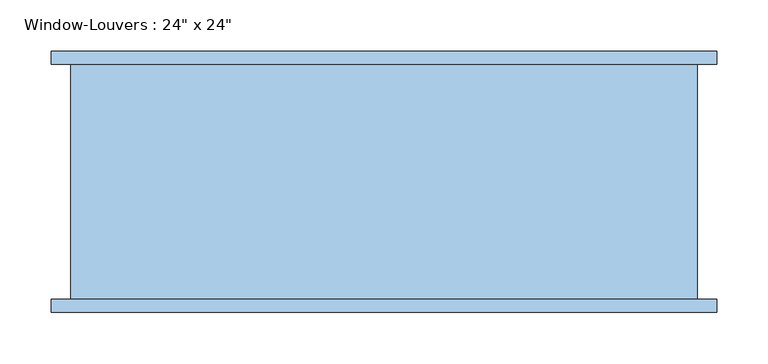
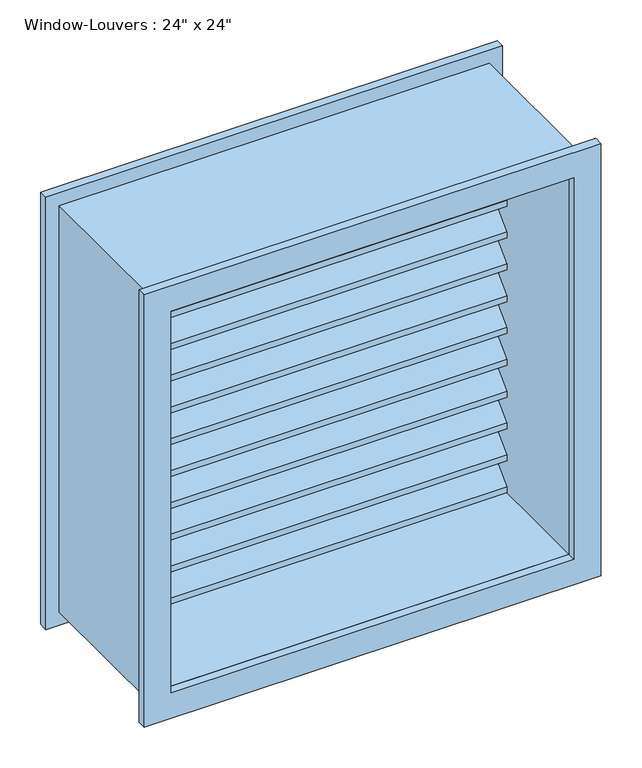
"""IFC4 building model written with IfcOpenShell, lengths in millimetres: window geometry."""

from ifc_helpers import new_model, si_unit, frame, origin, place, context, project, spatial, polyline, outline, extrude, source, transform, mapped, element, save


def window_f2d8fef0(model_context):
    return source(origin(), model_context, "Body", "SweptSolid", [
        extrude(outline(polyline([(107.95, 1419.1754778), (107.95, 1410.1952217), (69.85, 1448.2952217), (31.75, 1410.1952217), (31.75, 1419.1754778), (69.85, 1457.2754778), (107.95, 1419.1754778)])), frame((-285.75, 0.0, 0.0), z_axis=(1.0, 0.0, 0.0), x_axis=(0.0, 1.0, 0.0)), (0.0, 0.0, 1.0), 571.5),
        extrude(outline(polyline([(107.95, 1371.5009557), (107.95, 1362.5206995), (69.85, 1400.6206995), (31.75, 1362.5206995), (31.75, 1371.5009557), (69.85, 1409.6009557), (107.95, 1371.5009557)])), frame((-285.75, 0.0, 0.0), z_axis=(1.0, 0.0, 0.0), x_axis=(0.0, 1.0, 0.0)), (0.0, 0.0, 1.0), 571.5),
        extrude(outline(polyline([(107.95, 1323.8264335), (107.95, 1314.8461774), (69.85, 1352.9461774), (31.75, 1314.8461774), (31.75, 1323.8264335), (69.85, 1361.9264335), (107.95, 1323.8264335)])), frame((-285.75, 0.0, 0.0), z_axis=(1.0, 0.0, 0.0), x_axis=(0.0, 1.0, 0.0)), (0.0, 0.0, 1.0), 571.5),
        extrude(outline(polyline([(107.95, 1276.1519113), (107.95, 1267.1716552), (69.85, 1305.2716552), (31.75, 1267.1716552), (31.75, 1276.1519113), (69.85, 1314.2519113), (107.95, 1276.1519113)])), frame((-285.75, 0.0, 0.0), z_axis=(1.0, 0.0, 0.0), x_axis=(0.0, 1.0, 0.0)), (0.0, 0.0, 1.0), 571.5),
        extrude(outline(polyline([(107.95, 1228.4773891), (107.95, 1219.497133), (69.85, 1257.597133), (31.75, 1219.497133), (31.75, 1228.4773891), (69.85, 1266.5773891), (107.95, 1228.4773891)])), frame((-285.75, 0.0, 0.0), z_axis=(1.0, 0.0, 0.0), x_axis=(0.0, 1.0, 0.0)), (0.0, 0.0, 1.0), 571.5),
        extrude(outline(polyline([(107.95, 1180.802867), (107.95, 1171.8226109), (69.85, 1209.9226109), (31.75, 1171.8226109), (31.75, 1180.802867), (69.85, 1218.902867), (107.95, 1180.802867)])), frame((-285.75, 0.0, 0.0), z_axis=(1.0, 0.0, 0.0), x_axis=(0.0, 1.0, 0.0)), (0.0, 0.0, 1.0), 571.5),
        extrude(outline(polyline([(107.95, 1133.1283448), (107.95, 1124.1480887), (69.85, 1162.2480887), (31.75, 1124.1480887), (31.75, 1133.1283448), (69.85, 1171.2283448), (107.95, 1133.1283448)])), frame((-285.75, 0.0, 0.0), z_axis=(1.0, 0.0, 0.0), x_axis=(0.0, 1.0, 0.0)), (0.0, 0.0, 1.0), 571.5),
        extrude(outline(polyline([(107.95, 1085.4538226), (107.95, 1076.4735665), (69.85, 1114.5735665), (31.75, 1076.4735665), (31.75, 1085.4538226), (69.85, 1123.5538226), (107.95, 1085.4538226)])), frame((-285.75, 0.0, 0.0), z_axis=(1.0, 0.0, 0.0), x_axis=(0.0, 1.0, 0.0)), (0.0, 0.0, 1.0), 571.5),
        extrude(outline(polyline([(107.95, 1037.7793005), (107.95, 1028.7990443), (69.85, 1066.8990443), (31.75, 1028.7990443), (31.75, 1037.7793005), (69.85, 1075.8793005), (107.95, 1037.7793005)])), frame((-285.75, 0.0, 0.0), z_axis=(1.0, 0.0, 0.0), x_axis=(0.0, 1.0, 0.0)), (0.0, 0.0, 1.0), 571.5),
        extrude(outline(polyline([(107.95, 990.1047783), (107.95, 981.1245222), (69.85, 1019.2245222), (31.75, 981.1245222), (31.75, 990.1047783), (69.85, 1028.2047783), (107.95, 990.1047783)])), frame((-285.75, 0.0, 0.0), z_axis=(1.0, 0.0, 0.0), x_axis=(0.0, 1.0, 0.0)), (0.0, 0.0, 1.0), 571.5),
        extrude(outline(polyline([(107.95, 1466.85), (107.95, 1457.8697439), (69.85, 1495.9697439), (31.75, 1457.8697439), (31.75, 1466.85), (69.85, 1504.95), (107.95, 1466.85)])), frame((-285.75, 0.0, 0.0), z_axis=(1.0, 0.0, 0.0), x_axis=(0.0, 1.0, 0.0)), (0.0, 0.0, 1.0), 571.5),
        extrude(outline(polyline([(107.95, 942.4302561), (107.95, 933.45), (69.85, 971.55), (31.75, 933.45), (31.75, 942.4302561), (69.85, 980.5302561), (107.95, 942.4302561)])), frame((-285.75, 0.0, 0.0), z_axis=(1.0, 0.0, 0.0), x_axis=(0.0, 1.0, 0.0)), (0.0, 0.0, 1.0), 571.5),
        extrude(outline(polyline([(1524.0, 304.8), (1524.0, -304.8), (914.4, -304.8), (914.4, 304.8), (1524.0, 304.8)]), holes=[polyline([(1504.95, 285.75), (933.45, 285.75), (933.45, -285.75), (1504.95, -285.75), (1504.95, 285.75)])]), frame((0.0, -120.65, 0.0), z_axis=(0.0, 1.0, 0.0), x_axis=(0.0, 0.0, 1.0)), (0.0, 0.0, 1.0), 228.6),
        extrude(outline(polyline([(1543.05, 323.85), (1543.05, -323.85), (895.35, -323.85), (895.35, 323.85), (1543.05, 323.85)]), holes=[polyline([(1504.95, 285.75), (933.45, 285.75), (933.45, -285.75), (1504.95, -285.75), (1504.95, 285.75)])]), frame((0.0, -133.35, 0.0), z_axis=(0.0, 1.0, 0.0), x_axis=(0.0, 0.0, 1.0)), (0.0, 0.0, 1.0), 12.7),
        extrude(outline(polyline([(1543.05, -323.85), (895.35, -323.85), (895.35, 323.85), (1543.05, 323.85), (1543.05, -323.85)]), holes=[polyline([(1504.95, -285.75), (1504.95, 285.75), (933.45, 285.75), (933.45, -285.75), (1504.95, -285.75)])]), frame((0.0, 107.95, 0.0), z_axis=(0.0, 1.0, 0.0), x_axis=(0.0, 0.0, 1.0)), (0.0, 0.0, 1.0), 12.7),
    ])


if __name__ == "__main__":
    model = new_model("IFC4")
    model_context = context("Model", 3, world=origin())
    ifc_project = project(units=[si_unit("LENGTHUNIT", "METRE", prefix="MILLI")], contexts=[model_context])
    site = spatial("IfcSite", under=ifc_project)
    building = spatial("IfcBuilding", under=site)
    placement = place(None, origin())
    window_shape = window_f2d8fef0(model_context)
    element("IfcWindow", 1, ObjectType="Window-Louvers : 24\" x 24\"", at=placement, inside=building, context=model_context, shape_type="MappedRepresentation", body=[
        mapped(window_shape, transform((0.0, 0.0, 0.0), x_axis=(1.0, 0.0, 0.0), y_axis=(0.0, 1.0, 0.0), z_axis=(0.0, 0.0, 1.0))),
    ])
    save(model, "model.ifc")

# Revit data of these elements
# Type "Window-Louvers : 24\" x 24\""
#   Type Mark = "28"
#   Construction Type Id = "GSP4R"
#   Assembly Code = "B20"
#   Analytic Construction = "1/8 in Pilkington single glazing"
#   Visual Light Transmittance = 0.9
#   Thermal Resistance (R) = 0.271106 (m²·K)/W
#   Solar Heat Gain Coefficient = 0.78
#   Max Height = 1.978553 ft
#   Height = 2.0 ft
#   Heat Transfer Coefficient (U) = 3.6886 W/(m²·K)
#   Blade Width [instance default] = 1.875 ft
#   Blade Vertical Thickness = 0.029463 ft
#   Blade Thickness = 0.020833 ft
#   Blade Spacing = 0.125 ft
#   Blade Height = 0.154463 ft
#   Blade Depth = 0.25 ft
#   Blade Angle = 45.00°
#   Default Sill Height = 3.0 ft
#   Trim Projection_Exterior = 0.041667 ft
#   Trim Projection_Interior = 0.041667 ft
#   Trim Width_Exterior = 0.125 ft
#   Trim Width_Interior = 0.125 ft
#   Width = 2.0 ft
#   Max Blade Count = 12
#   Define Thermal Properties by = 1
#   Blade Count = 12
#   Frame Material = Birch
#   Louver Material = Birch
#   Trim Exterior Material = Birch
#   Trim Interior Material = Birch
#   Wall Closure = (empty or 0)
# Element 1 (IfcWindow, "Window-Louvers : 24\" x 24\"")
#   Materials on its faces: "Birch"
# Materials
#   "Birch": class "Wood", colour RGB 224 178 126, transparency 0, Description = "Betula Alleghaniensis", Cost = 0
